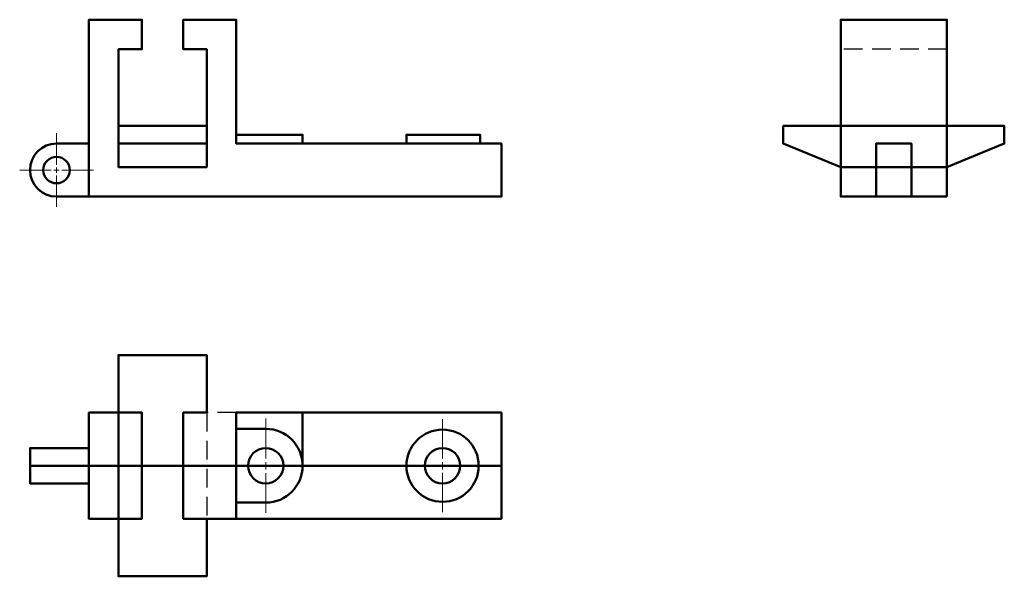
# Model space of a CAD drawing. Units: millimetres. Extents: x 21 to 355, y 78 to 267.
import ezdxf

# ---------------------------------------------------------------- set-up
doc = ezdxf.new("R2010")
doc.units = ezdxf.units.MM
doc.linetypes.add('CENTER', pattern=[50.8, 31.75, -6.35, 6.35, -6.35])
doc.linetypes.add('HIDDEN', pattern=[9.525, 6.35, -3.175])
for name, color, linetype, lineweight in [('M-CNTR', 1, 'CENTER', 18), ('M-HIDN', 3, 'HIDDEN', 25), ('M-OUTL', 7, 'Continuous', 50)]:
    doc.layers.add(name, color=color, linetype=linetype, lineweight=lineweight)

# ---------------------------------------------------------------- blocks, each defined once
blk = doc.blocks.new('*U1')
at = {"layer": 'M-CNTR', "color": 0, "transparency": 16777216}
for p, q in [((0, 1.8), (0, 12.5)), ((-12.5, 0), (-1.8, 0)), ((1.8, 0), (12.5, 0)), ((0, -12.5), (0, -1.8))]:
    blk.add_line(p, q, dxfattribs=at)
at = {"layer": 'M-CNTR', "color": 0, "linetype": 'Continuous', "transparency": 16777216}
for p, q in [((-0.9, 0), (0.9, 0)), ((0, -0.9), (0, 0.9))]:
    blk.add_line(p, q, dxfattribs=at)
blk = doc.blocks.new('*U2')
at = {"layer": 'M-CNTR', "color": 0, "transparency": 16777216}
for p, q in [((0, 2.5), (0, 16)), ((-16, 0), (-2.5, 0)), ((2.5, 0), (16, 0)), ((0, -16), (0, -2.5))]:
    blk.add_line(p, q, dxfattribs=at)
at = {"layer": 'M-CNTR', "color": 0, "linetype": 'Continuous', "transparency": 16777216}
for p, q in [((-1.25, 0), (1.25, 0)), ((0, -1.25), (0, 1.25))]:
    blk.add_line(p, q, dxfattribs=at)
blk = doc.blocks.new('*U3')
at = {"layer": 'M-CNTR', "color": 0, "transparency": 16777216}
for p, q in [((0, 2.45), (0, 15.75)), ((-15.75, 0), (-2.45, 0)), ((2.45, 0), (15.75, 0)), ((0, -15.75), (0, -2.45))]:
    blk.add_line(p, q, dxfattribs=at)
at = {"layer": 'M-CNTR', "color": 0, "linetype": 'Continuous', "transparency": 16777216}
for p, q in [((-1.225, 0), (1.225, 0)), ((0, -1.225), (0, 1.225))]:
    blk.add_line(p, q, dxfattribs=at)

msp = doc.modelspace()

# ---------------------------------------------------------------- linework, layer by layer
at = {"layer": 'M-HIDN'}
msp.add_line((335.38, 256.99), (299.38, 256.99), dxfattribs=at)
msp.add_lwpolyline([(94.23, 133.71), (84.23, 133.71), (84.23, 93.2)], dxfattribs=at)
at = {"layer": 'M-OUTL'}
for p, q in [((54.23, 230.99), (84.23, 230.99)), ((54.23, 224.99), (84.23, 224.99)), ((116.73, 133.71), (116.73, 115.71))]:
    msp.add_line(p, q, dxfattribs=at)
for points in [[(44.23, 224.99), (33.23, 224.99, 1), (33.23, 206.99), (44.23, 206.99), (44.23, 266.99), (62.23, 266.99), (62.23, 256.99), (54.23, 256.99), (54.23, 216.99), (84.23, 216.99), (84.23, 256.99), (76.23, 256.99), (76.23, 266.99), (94.23, 266.99), (94.23, 224.99), (184.23, 224.99), (184.23, 206.99), (44.23, 206.99)], [(94.23, 128.21), (104.23, 128.21, -1), (104.23, 103.21), (94.23, 103.21)]]:
    msp.add_lwpolyline(points, format="xyb", dxfattribs=at)
for points in [[(335.38, 206.99), (335.38, 266.99), (299.38, 266.99), (299.38, 206.99)], [(299.38, 230.99), (335.38, 230.99), (354.88, 230.99), (354.88, 224.99), (335.38, 216.99), (299.38, 216.99), (279.88, 224.99), (279.88, 230.99)]]:
    msp.add_lwpolyline(points, close=True, dxfattribs=at)
for points in [[(94.23, 227.99), (116.73, 227.99), (116.73, 224.99)], [(151.98, 224.99), (151.98, 227.99), (176.98, 227.99), (176.98, 224.99)], [(311.38, 206.99), (311.38, 224.99), (323.38, 224.99), (323.38, 206.99)], [(94.23, 97.71), (184.23, 97.71), (184.23, 133.71), (94.23, 133.71), (94.23, 97.71), (84.23, 97.71), (76.23, 97.71), (76.23, 133.71), (84.23, 133.71), (84.23, 153.21), (54.23, 153.21), (54.23, 133.71), (54.23, 97.71), (62.23, 97.71), (62.23, 133.71), (54.23, 133.71), (44.23, 133.71), (44.23, 97.71), (52.48, 97.71)], [(24.23, 115.71), (24.23, 121.71), (44.23, 121.71)], [(184.23, 115.71), (44.23, 115.71), (24.23, 115.71), (24.23, 109.71), (44.23, 109.71)], [(50.73, 97.71), (54.23, 97.71), (54.23, 78.21), (84.23, 78.21), (84.23, 97.71)]]:
    msp.add_lwpolyline(points, dxfattribs=at)
for centre, radius in [((33.23, 215.99), 4.5), ((164.23, 115.71), 12.25), ((104.23, 115.71), 6), ((164.23, 115.71), 6)]:
    msp.add_circle(centre, radius, dxfattribs=at)

# ---------------------------------------------------------------- block references
at = {"layer": 'M-CNTR'}
for name, p in [('*U1', (33.23, 215.99)), ('*U2', (104.23, 115.71)), ('*U3', (164.23, 115.71))]:
    msp.add_blockref(name, p, dxfattribs=at)

doc.saveas('drawing.dxf')
